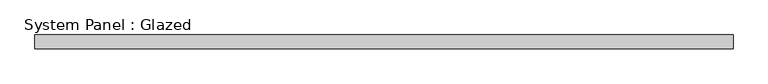
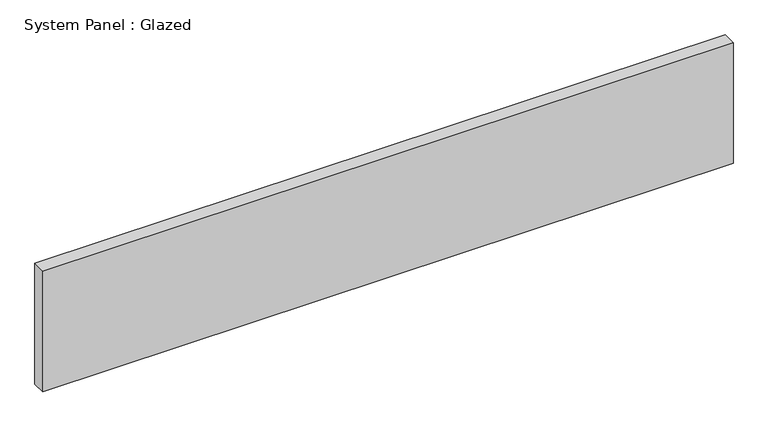
"""IFC4 building model written with IfcOpenShell, lengths in millimetres: plate geometry, System Panel : Glazed."""

from ifc_helpers import new_model, si_unit, origin, origin_with_axes, place, context, project, spatial, polyline, outline, extrude, source, transform, mapped, element, save


def system_panel_glazed_f096bff0(model_context):
    return source(origin(), model_context, "Body", "SweptSolid", [
        extrude(outline(polyline([(637.0528322, 19.05), (-637.0528322, 19.05), (-637.0528322, 44.45), (637.0528322, 44.45), (637.0528322, 19.05)])), origin_with_axes(), (0.0, 0.0, 1.0), 235.2097418),
    ])


if __name__ == "__main__":
    model = new_model("IFC4")
    model_context = context("Model", 3, world=origin())
    ifc_project = project(units=[si_unit("LENGTHUNIT", "METRE", prefix="MILLI")], contexts=[model_context])
    site = spatial("IfcSite", under=ifc_project)
    building = spatial("IfcBuilding", under=site)
    placement = place(None, origin())
    system_panel_glazed_shape = system_panel_glazed_f096bff0(model_context)
    element("IfcPlate", 1, ObjectType="System Panel : Glazed", at=placement, inside=building, context=model_context, shape_type="MappedRepresentation", body=[
        mapped(system_panel_glazed_shape, transform((0.0, 0.0, 0.0), x_axis=(1.0, 0.0, 0.0), y_axis=(0.0, 1.0, 0.0), z_axis=(0.0, 0.0, 1.0))),
    ])
    save(model, "model.ifc")

# Revit data of these elements
# Type "System Panel : Glazed"
#   Construction Type Id = "GSP4R"
#   Analytic Construction = "1/8 in Pilkington single glazing"
#   Visual Light Transmittance = 0.9
#   Solar Heat Gain Coefficient = 0.86
#   Heat Transfer Coefficient (U) = 1.18115 BTU/(h·ft²·°F)
#   Define Thermal Properties by = 1
# Element 1 (IfcPlate, "System Panel : Glazed")
#   Materials on its faces: "Glass"
# Materials
#   "Glass": class "Glass", colour RGB 0 128 192, transparency 0.75, Description = "Soda Lime Glass", Cost = 0
